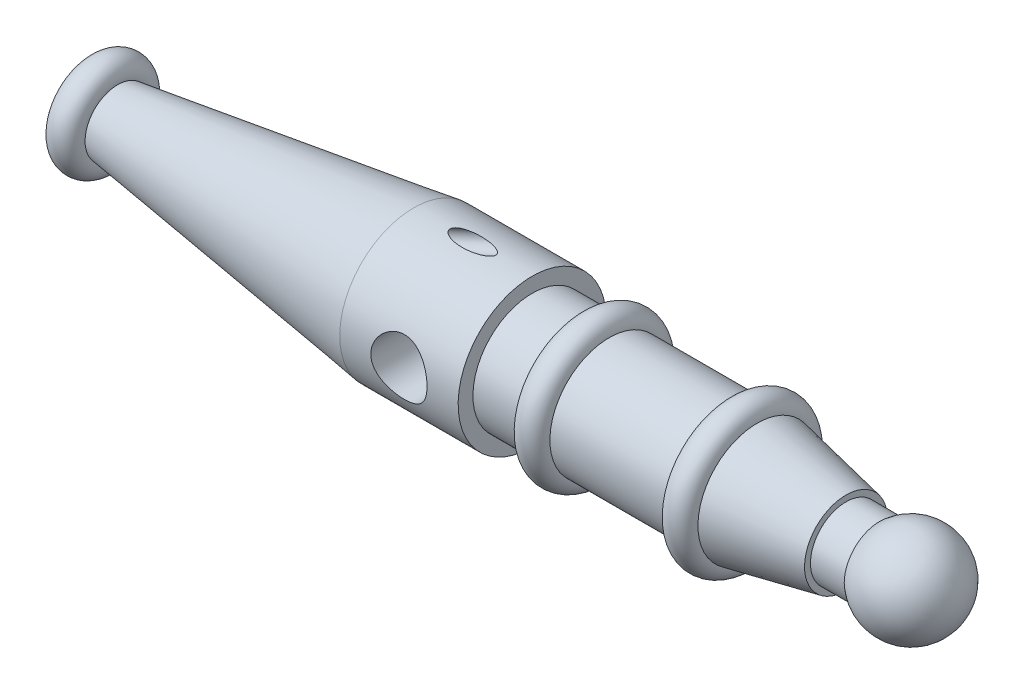
from build123d import *

# Parameters (mm, degrees)
BORE_SKETCH_64_R              = 32
BORE_64_X375_DEPTH            = 375
BORE_MOUTH_CHAMFER_16X45_SIZE = 16
CROSS_HOLE_CUT_DEPTH          = 813.545629788
CROSS_HOLE_CUT_DEPTH_BACK     = 813.545629788
CROSS_HOLE_SKETCH_R           = 47.5
DEEP_BORE_SKETCH_R            = 32
DEEP_BORE_CUT_555_DEPTH       = 555


with BuildPart() as part:
    # Body Profile Sketch → Revolved Body (revolve)
    with BuildSketch(Plane.XY, mode=Mode.PRIVATE) as revolved_body_sk:
        with BuildLine():
            Line((-676.832180336, 55), (-676.832180336, 0))
            Line((-676.832180336, 0), (793.082845885, 0))
            ThreePointArc((793.082845885, 0), (745.997872106, 72.915026221), (660.167819664, 60))
            Line((660.167819664, 60), (603.167819664, 60))
            Line((603.167819664, 60), (603.167819664, 70))
            Line((603.167819664, 70), (453.167819664, 100))
            ThreePointArc((453.167819664, 100), (428.167819664, 125), (403.167819664, 100))
            Line((403.167819664, 100), (203.167819664, 100))
            ThreePointArc((203.167819664, 100), (178.167819664, 125), (153.167819664, 100))
            Line((153.167819664, 100), (73.167819664, 100))
            Line((73.167819664, 100), (73.167819664, 125))
            Line((73.167819664, 125), (-126.832180336, 125))
            Line((-126.832180336, 125), (-626.832180336, 55))
            ThreePointArc((-626.832180336, 55), (-651.832180336, 85.495097568), (-676.832180336, 55))
        make_face()
    revolve(revolved_body_sk.sketch.rotate(Axis((-676.832180336, 0, 0), (1, 0, 0)), 180), axis=Axis((-676.832180336, 0, 0), (1, 0, 0)))

    # Bore Sketch Ø64 → Bore Ø64 x375 (cut)
    with BuildSketch(Plane.ZY.offset(676.832180336)):
        with Locations(Location((0, 0, 0), (0, 0, 270))):
            Circle(BORE_SKETCH_64_R)
    extrude(amount=-BORE_64_X375_DEPTH, mode=Mode.SUBTRACT)

    # Bore Mouth Chamfer 16x45
    bore_mouth_chamfer_16x45_edges = [part.edges().sort_by_distance(p)[0] for p in [
        (-676.832180336, 32, 0),
    ]]
    chamfer(bore_mouth_chamfer_16x45_edges, length=BORE_MOUTH_CHAMFER_16X45_SIZE)

    # Cross Hole Sketch → Cross Hole Cut (cut, two sides: drawn at the far end of the back side and taken through both)
    with BuildSketch(Plane.XY.offset(-CROSS_HOLE_CUT_DEPTH_BACK)):
        with Locations((-26.832180336, 0)):
            Circle(CROSS_HOLE_SKETCH_R)
    extrude(amount=CROSS_HOLE_CUT_DEPTH + CROSS_HOLE_CUT_DEPTH_BACK, mode=Mode.SUBTRACT)

    # Groove Profile Sketch → Revolved Groove Cut (revolve, cut)
    with BuildSketch(Plane.XY, mode=Mode.PRIVATE) as revolved_groove_cut_sk:
        Polygon((-350.038031958, -5.086668407), (-343.388613806, -19.639511367), (28.843028109, 150.438860479), (22.193609957, 164.99170344), align=None)
    revolve(revolved_groove_cut_sk.sketch.rotate(Axis((-343.388613806, -19.639511367, 0), (0.9095526850462128, 0.41558863449957945, 0)), 180), axis=Axis((-343.388613806, -19.639511367, 0), (0.9095526850462128, 0.41558863449957945, 0)), mode=Mode.SUBTRACT)

    # Deep Bore Sketch → Deep Bore Cut 555 (cut)
    with BuildSketch(Plane.ZY.offset(676.832180336)):
        with Locations(Location((0, 0, 0), (0, 0, 270))):
            Circle(DEEP_BORE_SKETCH_R)
    extrude(amount=-DEEP_BORE_CUT_555_DEPTH, mode=Mode.SUBTRACT)


solid = part.part
